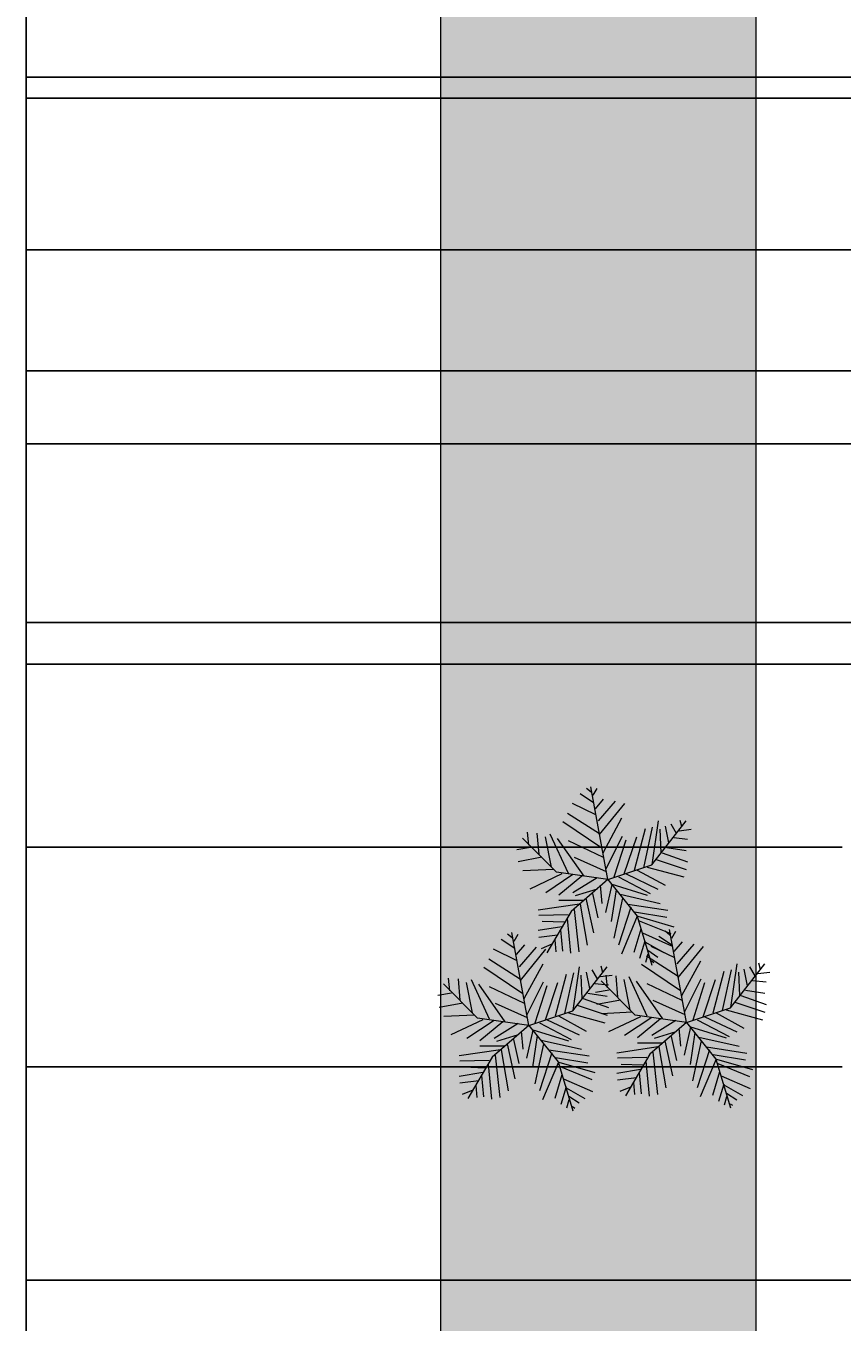
# Model space of a CAD drawing. Units: millimetres. Extents: x -229 to 16545, y -10488 to 4272.
# Tile 2 of 29: x -229 to 2016, y -4633 to -1067. Entities that reach past the tile are written whole.
import ezdxf

# ---------------------------------------------------------------- set-up
doc = ezdxf.new("R2010")
doc.units = ezdxf.units.MM
for name, color, linetype, lineweight in [('A-ANNO-DIMS', 2, 'Continuous', 18), ('L-PLNT-BEDS', 82, 'Continuous', 18), ('L-PLNT-TREE', 80, 'Continuous', 18)]:
    doc.layers.add(name, color=color, linetype=linetype, lineweight=lineweight)
doc.layers.add('L-PLNT-PATT', color=116, linetype='Continuous', lineweight=13, true_color=0x136734)
doc.styles.get("Standard").update_dxf_attribs({"font": 'arial.ttf'})
doc.dimstyles.get("Standard").update_dxf_attribs({"dimtxt": 0.18, "dimasz": 0.18, "dimexe": 0.18, "dimexo": 0.0625, "dimgap": 0.09, "dimtad": 0, "dimtih": 1, "dimtoh": 1, "dimdec": 4, "dimzin": 0, "dimdsep": 46, "dimtxsty": 'Standard', "dimcen": 0.09, "dimadec": 0, "dimazin": 0, "dimtfac": 1, "dimtdec": 4, "dimtofl": 0, "dimtmove": 0, "dimatfit": 3, "dimfxl": 1, "dimtolj": 1, "dimtzin": 0, "dimarcsym": 0})

# ---------------------------------------------------------------- blocks, each defined once
blk = doc.blocks.new('*U18')
for p, q in [((-10.186, 53.64), (-13.084, 55.962)), ((0, 0), (-10.5, 57)), ((-9.099, 51.782), (-6.563, 55.962)), ((-8.737, 47.138), (-17.069, 52.711)), ((-7.65, 43.423), (-2.578, 49.46)), ((-5.839, 35.992), (4.667, 48.067)), ((-5.114, 28.097), (-24.676, 40.636)), ((-7.288, 39.707), (-21.778, 46.673)), ((-5.114, 27.632), (10.463, 46.673)), ((-3.665, 19.273), (-27.574, 35.527)), ((-2.941, 16.486), (8.652, 37.85)), ((22.055, 7.198), (27.489, 32.277)), ((27, 9), (48, 36)), ((27.127, 9.056), (31.112, 35.992)), ((35.096, 32.741), (37.27, 22.524)), ((38.719, 34.134), (41.979, 28.561)), ((44.153, 36.456), (45.239, 32.741)), ((-31.5, 4.5), (-52.5, 25.5)), ((-48.585, 21.131), (-49.309, 29.026)), ((-43.513, 28.561), (-42.427, 15.558)), ((-38.442, 26.239), (-34.819, 7.663)), ((-35.544, 28.097), (-24.314, 3.947)), ((-14.533, 2.09), (-30.834, 25.31)), ((-24.314, 23.917), (-2.941, 13.7)), ((-1.129, 6.734), (9.014, 26.704)), ((3.942, 1.625), (11.187, 24.381)), ((10.101, 3.483), (17.708, 26.239)), ((16.259, 5.805), (23.142, 31.348)), ((31.836, 30.883), (32.561, 16.486)), ((40.53, 25.775), (48.862, 24.846)), ((43.791, 29.954), (51.036, 30.883)), ((-47.498, 19.737), (-55.83, 18.344)), ((33.285, 16.486), (48.862, 10.913)), ((36.183, 19.737), (48.137, 17.88)), ((-40.615, 13.7), (-55.105, 10.913)), ((-20.691, 13.7), (-1.129, 4.876)), ((0, 0), (27, 9)), ((29.662, 12.307), (48.137, 6.269)), ((-33.37, 6.269), (-52.207, 5.34)), ((-28.299, 3.483), (-47.86, -5.805)), ((-21.416, 3.018), (-38.079, -8.128)), ((0, 0), (-31.5, 4.5)), ((-15.982, 2.09), (-30.11, -9.521)), ((0, 0), (-22.5, -19.5)), ((-6.563, 1.161), (-21.416, -8.128)), ((0, 0), (18, -22.5)), ((6.478, 1.625), (26.04, -8.592)), ((11.187, 3.483), (30.749, -5.805)), ((18.07, 5.805), (35.096, -3.483)), ((24.229, 7.663), (46.688, 1.625)), ((-6.563, -5.805), (-19.967, -9.985)), ((-4.752, -3.483), (-3.665, -14.629)), ((2.493, -3.019), (-1.491, -20.202)), ((1.769, -2.555), (24.229, -9.521)), ((5.029, -6.27), (2.131, -25.775)), ((-17.431, -15.094), (-42.789, -18.809)), ((-15.257, -12.772), (-30.11, -12.772)), ((-17.069, -15.094), (-12.721, -40.172)), ((-13.446, -11.378), (-8.737, -32.741)), ((-9.461, -8.592), (-6.201, -23.453)), ((9.014, -11.378), (3.58, -35.992)), ((7.565, -9.056), (32.198, -14.629)), ((12.274, -15.094), (36.907, -18.809)), ((-24.314, -21.596), (-42.427, -22.06)), ((-22.5, -19.5), (-37.5, -45)), ((-20.691, -18.345), (-17.793, -44.352)), ((14.085, -16.951), (6.478, -40.172)), ((18.07, -22.524), (8.289, -45.745)), ((16.259, -19.738), (36.183, -22.989)), ((18, -22.5), (27, -52.5)), ((18.433, -22.524), (40.53, -29.026)), ((-28.299, -29.026), (-42.789, -31.348)), ((-26.849, -26.24), (-40.253, -25.775)), ((-29.023, -30.884), (-27.936, -43.887)), ((-25.038, -23.918), (-22.865, -45.281)), ((20.244, -30.419), (15.897, -44.816)), ((19.157, -25.311), (38.719, -33.206)), ((-30.834, -34.135), (-42.427, -35.528)), ((-34.457, -39.708), (-40.978, -42.494)), ((-32.646, -36.921), (-31.921, -44.352)), ((22.78, -37.85), (19.519, -48.532)), ((21.331, -32.741), (39.081, -40.636)), ((22.78, -38.314), (34.372, -44.816)), ((24.591, -45.745), (23.142, -50.854)), ((24.591, -43.423), (30.749, -47.603)), ((26.764, -49.925), (28.213, -50.854))]:
    blk.add_line(p, q)
blk = doc.blocks.new('*D46')
at = {"layer": 'A-ANNO-DIMS', "color": 0, "lineweight": -2, "transparency": 16777216}
for p, q in [((912, 2251.7), (-228.8, 2251.7)), ((-228.7, 2251.5), (-228.7, -3498.1)), ((-228.7, -9248.1), (-228.7, -3498.5)), ((912, -9248.3), (-228.8, -9248.3))]:
    blk.add_line(p, q, dxfattribs=at)
at = {"layer": 'A-ANNO-DIMS', "color": 0, "transparency": 16777216}
for points in [[(-228.7, 2251.5), (-228.6, 2251.5), (-228.7, 2251.7)], [(-228.7, -9248.1), (-228.6, -9248.1), (-228.7, -9248.3)]]:
    blk.add_solid(points, dxfattribs=at)
at = {"layer": 'Defpoints', "color": 0, "transparency": 16777216}
for p in [(912.1, 2251.7), (-228.7, -9248.3), (912.1, -9248.3)]:
    blk.add_point(p, dxfattribs=at)
at = {"layer": 'A-ANNO-DIMS', "color": 0, "transparency": 16777216, "insert": (-228.7, -3498.3), "char_height": 0.18, "attachment_point": 5}
blk.add_mtext('\\A1;11500', dxfattribs=at)
blk = doc.blocks.new('*D55')
at = {"layer": 'A-ANNO-DIMS', "color": 0, "lineweight": -2, "transparency": 16777216}
for p, q in [((4445.9, -1208.3), (-228.8, -1208.3)), ((-228.7, -1208.5), (-228.7, -1958.1)), ((-228.7, -2708.1), (-228.7, -1958.5)), ((4445.9, -2708.3), (-228.8, -2708.3))]:
    blk.add_line(p, q, dxfattribs=at)
at = {"layer": 'A-ANNO-DIMS', "color": 0, "transparency": 16777216}
for points in [[(-228.7, -1208.5), (-228.6, -1208.5), (-228.7, -1208.3)], [(-228.7, -2708.1), (-228.6, -2708.1), (-228.7, -2708.3)]]:
    blk.add_solid(points, dxfattribs=at)
at = {"layer": 'Defpoints', "color": 0, "transparency": 16777216}
for p in [(4445.9, -1208.3), (-228.7, -2708.3), (4445.9, -2708.3)]:
    blk.add_point(p, dxfattribs=at)
at = {"layer": 'A-ANNO-DIMS', "color": 0, "transparency": 16777216, "insert": (-228.7, -1958.3), "char_height": 0.18, "attachment_point": 5}
blk.add_mtext('\\A1;1500', dxfattribs=at)
blk = doc.blocks.new('*D56')
at = {"layer": 'A-ANNO-DIMS', "color": 0, "lineweight": -2, "transparency": 16777216}
for p, q in [((2245.9, -2823.3), (-228.8, -2823.3)), ((-228.7, -2823.5), (-228.7, -3670.6)), ((-228.7, -4518.1), (-228.7, -3671)), ((2245.9, -4518.3), (-228.8, -4518.3))]:
    blk.add_line(p, q, dxfattribs=at)
at = {"layer": 'A-ANNO-DIMS', "color": 0, "transparency": 16777216}
for points in [[(-228.7, -2823.5), (-228.6, -2823.5), (-228.7, -2823.3)], [(-228.7, -4518.1), (-228.6, -4518.1), (-228.7, -4518.3)]]:
    blk.add_solid(points, dxfattribs=at)
at = {"layer": 'Defpoints', "color": 0, "transparency": 16777216}
for p in [(2245.9, -2823.3), (-228.7, -4518.3), (2245.9, -4518.3)]:
    blk.add_point(p, dxfattribs=at)
at = {"layer": 'A-ANNO-DIMS', "color": 0, "transparency": 16777216, "insert": (-228.7, -3670.8), "char_height": 0.18, "attachment_point": 5}
blk.add_mtext('\\A1;1695', dxfattribs=at)
blk = doc.blocks.new('*D73')
at = {"layer": 'A-ANNO-DIMS', "color": 0, "lineweight": -2, "transparency": 16777216}
for p, q in [((2015.9, -3326.8), (-228.8, -3326.8)), ((-228.7, -3327), (-228.7, -3628.7)), ((-228.7, -3930.9), (-228.7, -3629.1)), ((2015.9, -3931), (-228.8, -3931))]:
    blk.add_line(p, q, dxfattribs=at)
at = {"layer": 'A-ANNO-DIMS', "color": 0, "transparency": 16777216}
for points in [[(-228.7, -3327), (-228.6, -3327), (-228.7, -3326.8)], [(-228.7, -3930.9), (-228.6, -3930.9), (-228.7, -3931)]]:
    blk.add_solid(points, dxfattribs=at)
at = {"layer": 'Defpoints', "color": 0, "transparency": 16777216}
for p in [(2015.9, -3326.8), (-228.7, -3931), (2015.9, -3931)]:
    blk.add_point(p, dxfattribs=at)
at = {"layer": 'A-ANNO-DIMS', "color": 0, "transparency": 16777216, "insert": (-228.7, -3628.9), "char_height": 0.18, "attachment_point": 5}
blk.add_mtext('\\A1;604.2', dxfattribs=at)
blk = doc.blocks.new('*D83')
at = {"layer": 'A-ANNO-DIMS', "color": 0, "lineweight": -2, "transparency": 16777216}
for p, q in [((4448.4, -1265.8), (-228.8, -1265.8)), ((-228.7, -1266), (-228.7, -1640.6)), ((-228.7, -2015.6), (-228.7, -1641)), ((4445.9, -2015.8), (-228.8, -2015.8))]:
    blk.add_line(p, q, dxfattribs=at)
at = {"layer": 'A-ANNO-DIMS', "color": 0, "transparency": 16777216}
for points in [[(-228.7, -1266), (-228.6, -1266), (-228.7, -1265.8)], [(-228.7, -2015.6), (-228.6, -2015.6), (-228.7, -2015.8)]]:
    blk.add_solid(points, dxfattribs=at)
at = {"layer": 'Defpoints', "color": 0, "transparency": 16777216}
for p in [(4448.4, -1265.8), (-228.7, -2015.8), (4445.9, -2015.8)]:
    blk.add_point(p, dxfattribs=at)
at = {"layer": 'A-ANNO-DIMS', "color": 0, "transparency": 16777216, "insert": (-228.7, -1640.8), "char_height": 0.18, "attachment_point": 5}
blk.add_mtext('\\A1;750', dxfattribs=at)
blk = doc.blocks.new('*D88')
at = {"layer": 'A-ANNO-DIMS', "color": 0, "lineweight": -2, "transparency": 16777216}
for p, q in [((2015.9, -3931), (-228.8, -3931)), ((-228.7, -3931.2), (-228.7, -4224.5)), ((-228.7, -4518.1), (-228.7, -4224.8)), ((2245.9, -4518.3), (-228.8, -4518.3))]:
    blk.add_line(p, q, dxfattribs=at)
at = {"layer": 'A-ANNO-DIMS', "color": 0, "transparency": 16777216}
for points in [[(-228.7, -3931.2), (-228.6, -3931.2), (-228.7, -3931)], [(-228.7, -4518.1), (-228.6, -4518.1), (-228.7, -4518.3)]]:
    blk.add_solid(points, dxfattribs=at)
at = {"layer": 'Defpoints', "color": 0, "transparency": 16777216}
for p in [(2015.9, -3931), (-228.7, -4518.3), (2245.9, -4518.3)]:
    blk.add_point(p, dxfattribs=at)
at = {"layer": 'A-ANNO-DIMS', "color": 0, "transparency": 16777216, "insert": (-228.7, -4224.7), "char_height": 0.18, "attachment_point": 5}
blk.add_mtext('\\A1;587.2', dxfattribs=at)
blk = doc.blocks.new('*D94')
at = {"layer": 'A-ANNO-DIMS', "color": 0, "lineweight": -2, "transparency": 16777216}
for p, q in [((2283.9, -1683.5), (-228.8, -1683.5)), ((-228.7, -1683.7), (-228.7, -1950)), ((-228.7, -2216.7), (-228.7, -1950.4)), ((2283.9, -2216.9), (-228.8, -2216.9))]:
    blk.add_line(p, q, dxfattribs=at)
at = {"layer": 'A-ANNO-DIMS', "color": 0, "transparency": 16777216}
for points in [[(-228.7, -1683.7), (-228.6, -1683.7), (-228.7, -1683.5)], [(-228.7, -2216.7), (-228.6, -2216.7), (-228.7, -2216.9)]]:
    blk.add_solid(points, dxfattribs=at)
at = {"layer": 'Defpoints', "color": 0, "transparency": 16777216}
for p in [(2284, -1683.5), (-228.7, -2216.9), (2284, -2216.9)]:
    blk.add_point(p, dxfattribs=at)
at = {"layer": 'A-ANNO-DIMS', "color": 0, "transparency": 16777216, "insert": (-228.7, -1950.2), "char_height": 0.18, "attachment_point": 5}
blk.add_mtext('\\A1;533.4', dxfattribs=at)

msp = doc.modelspace()

# ---------------------------------------------------------------- hatches: boundary and pattern name
at = {"layer": 'L-PLNT-PATT'}
h = msp.add_hatch(dxfattribs=at)
h.set_pattern_fill('GRASS', color=256)
h.set_pattern_definition([(90, (-8141.222, -13125.504), (-17.960512, 17.960512), [4.7625, -31.158524]), (45, (-8141.222, -13125.504), (-17.960512, 17.960512), [4.7625, -20.6375]), (135, (-8141.222, -13125.504), (-17.960512, -17.960512), [4.7625, -20.6375])])
h.paths.add_polyline_path([(1778.331, 2251.728), (912.052, 2251.728), (912.052, -9248.272), (1778.331, -9248.272), (1914.943, -9248.272), (1914.943, -7879.258), (1778.331, -7879.258)])
h = msp.add_hatch(dxfattribs=at)
h.set_pattern_fill('GRASS', color=256, scale=5.9)
h.set_pattern_definition([(90, (-8141.22, -13125.5), (-105.967, 105.967), [28.0987, -183.8353]), (45, (-8141.22, -13125.5), (-105.967, 105.967), [28.0987, -121.7613]), (135, (-8141.22, -13125.5), (-105.967, -105.967), [28.0987, -121.7613])])
h.paths.add_polyline_path([(1778.331, 2251.728), (912.052, 2251.728), (912.052, -9248.272), (1778.331, -9248.272), (1914.943, -9248.272), (1914.943, -7879.258), (1778.331, -7879.258)])

# ---------------------------------------------------------------- linework, layer by layer
at = {"layer": 'L-PLNT-BEDS', "transparency": 33554554}
msp.add_line((912.052, -9248.272), (912.052, 2251.728), dxfattribs=at)
at = {"layer": 'L-PLNT-BEDS', "transparency": 33554569}
msp.add_line((1778.331, 2251.728), (1778.331, -7879.258), dxfattribs=at)

# ---------------------------------------------------------------- block references
at = {"layer": 'L-PLNT-TREE', "xscale": 4.481031954380777, "yscale": 4.481031954380777, "zscale": 4.481031954380777}
for p in [(1371.699, -3415.863), (1154.536, -3816.921), (1588.225, -3808.741)]:
    msp.add_blockref('*U18', p, dxfattribs=at)

# ---------------------------------------------------------------- dimensions: what is measured, and where the dimension line sits
at = {"layer": 'A-ANNO-DIMS'}
for base, p1, p2, override, picture, middle in [((-228.657, -9248.272), (912.052, 2251.728), (912.052, -9248.272), {"dimdec": 0, "dimlfac": 1, "dimrnd": 0, "dimzin": 0, "dimdsep": 46, "dimlunit": 2}, '*D46', (-228.657, -3498.272)), ((-228.657, -2708.272), (4445.933, -1208.272), (4445.933, -2708.272), {"dimdec": 0, "dimlfac": 1, "dimrnd": 0, "dimzin": 0, "dimdsep": 46, "dimlunit": 2}, '*D55', (-228.657, -1958.272)), ((-228.657, -2015.768), (4448.433, -1265.772), (4445.933, -2015.768), {"dimdec": 0, "dimlfac": 1, "dimrnd": 0, "dimzin": 0, "dimdsep": 46, "dimlunit": 2}, '*D83', (-228.657, -1640.77)), ((-228.657, -2216.899), (2284.002, -1683.499), (2284.002, -2216.899), {"dimdec": 1, "dimlfac": 1, "dimrnd": 0, "dimzin": 0, "dimdsep": 46, "dimlunit": 2}, '*D94', (-228.657, -1950.199)), ((-228.657, -4518.272), (2245.933, -2823.272), (2245.933, -4518.272), {"dimdec": 0, "dimlfac": 1, "dimrnd": 0, "dimzin": 0, "dimdsep": 46, "dimlunit": 2}, '*D56', (-228.657, -3670.772)), ((-228.657, -3931.042), (2015.933, -3326.811), (2015.933, -3931.042), {"dimdec": 1, "dimlfac": 1, "dimrnd": 0, "dimzin": 0, "dimdsep": 46, "dimlunit": 2}, '*D73', (-228.657, -3628.926)), ((-228.657, -4518.272), (2015.933, -3931.042), (2245.933, -4518.272), {"dimdec": 1, "dimlfac": 1, "dimrnd": 0, "dimzin": 0, "dimdsep": 46, "dimlunit": 2}, '*D88', (-228.657, -4224.657))]:
    dim = msp.add_linear_dim(base=base, p1=p1, p2=p2, angle=90, dimstyle='Standard', override=override, dxfattribs=at)
    dim.commit()
    dim.dimension.update_dxf_attribs({"geometry": picture, "text_midpoint": middle})

doc.saveas('drawing.dxf')
